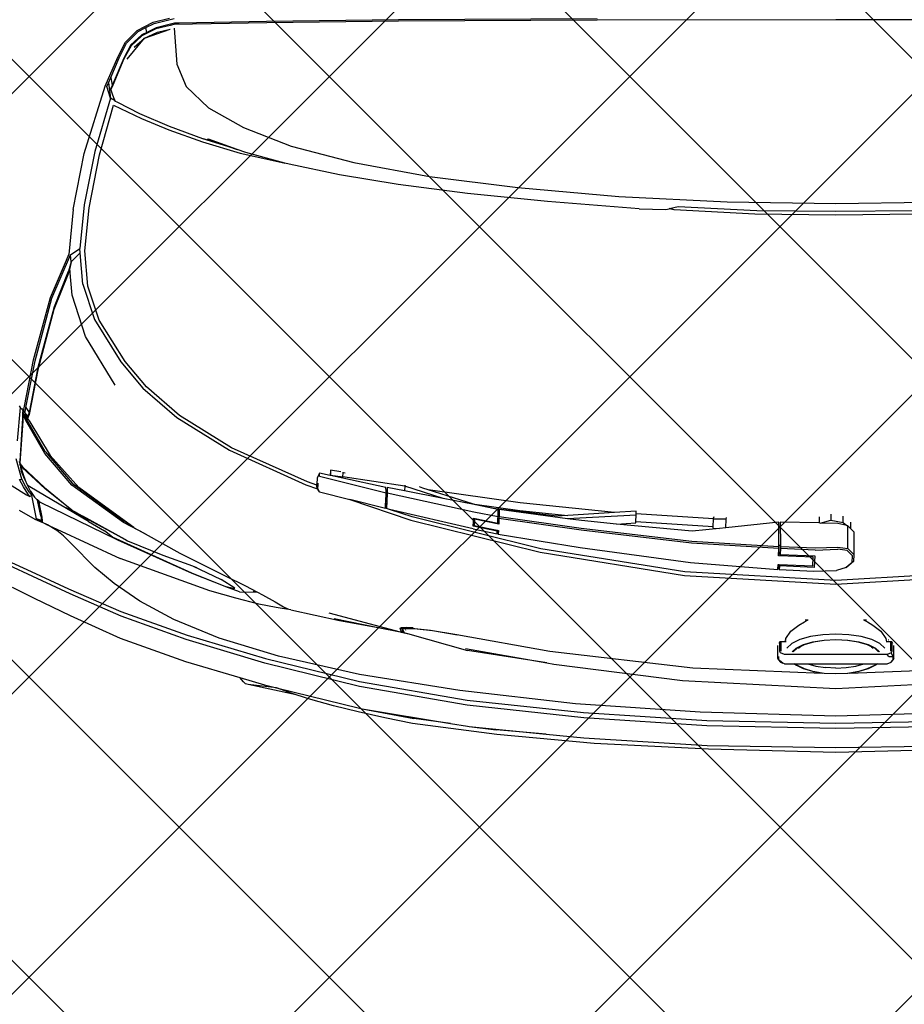
# Model space of a CAD drawing. Units: inches. Extents: x 2167 to 2589, y 1680 to 2489.
# Tile 4 of 38: x 2262.53 to 2283.35, y 1703.49 to 1726.68. Entities that reach past the tile are written whole.
import ezdxf

# ---------------------------------------------------------------- set-up
doc = ezdxf.new("R2010")
doc.units = ezdxf.units.IN
doc.header["$MEASUREMENT"] = 0
doc.layers.get('0').update_dxf_attribs({"color": 250})
for name, color, linetype, lineweight in [('A-ANNO-DIMS', 2, 'Continuous', 18), ('C-PRKG-VEHS', 8, 'Continuous', 13), ('L-PVMT-PATT', 252, 'Continuous', 13)]:
    doc.layers.add(name, color=color, linetype=linetype, lineweight=lineweight)
doc.layers.add('Edges', color=250, linetype='Continuous')
doc.styles.get("Standard").update_dxf_attribs({"font": 'arial.ttf'})
doc.dimstyles.get("Standard").update_dxf_attribs({"dimtxt": 7, "dimasz": 0.18, "dimexe": 0.18, "dimexo": 0.0625, "dimgap": 0.09, "dimtad": 0, "dimtih": 1, "dimtoh": 1, "dimdec": 1, "dimzin": 0, "dimdsep": 46, "dimlunit": 3, "dimtxsty": 'Standard', "dimcen": 0.09, "dimadec": 0, "dimazin": 0, "dimtfac": 1, "dimtdec": 1, "dimtofl": 0, "dimtmove": 0, "dimatfit": 3, "dimfxl": 1, "dimtolj": 1, "dimtzin": 0, "dimarcsym": 0})

# ---------------------------------------------------------------- blocks, each defined once
blk = doc.blocks.new('Nissan Qashqai pl')
at = {"layer": 'Edges'}
for p, q in [((11.05972, 12.11965), (11.05938, 11.92208)), ((11.5166, 12.04708), (11.52386, 11.92208)), ((11.52698, 11.92208), (11.51964, 12.0475)), ((11.61327, 11.92208), (11.60675, 12.04892)), ((11.60051, 11.93346), (11.59629, 12.04057)), ((11.63292, 12.0344), (11.63628, 11.92208)), ((11.64211, 11.92208), (11.63993, 12.02899)), ((11.64437, 12.02886), (11.64655, 11.92208)), ((11.66226, 11.92208), (11.66041, 12.02874)), ((11.66349, 12.02738), (11.66628, 11.92208)), ((11.21164, 11.92208), (11.21014, 12.01197)), ((11.21801, 11.92208), (11.21745, 11.98742)), ((11.22044, 11.98904), (11.22108, 11.92208)), ((11.57261, 11.96533), (11.57261, 11.96561)), ((11.57306, 11.96528), (11.57306, 11.96569)), ((11.57479, 11.96843), (11.57457, 11.96768)), ((11.58239, 11.96768), (11.57457, 11.96768)), ((11.57457, 11.96768), (11.57457, 11.96395)), ((11.57617, 11.96938), (11.57479, 11.96843)), ((11.57479, 11.96843), (11.58262, 11.96843)), ((11.58846, 11.97008), (11.57758, 11.97008)), ((11.58262, 11.96843), (11.58377, 11.96782)), ((11.58668, 11.96947), (11.58377, 11.96782)), ((11.58377, 11.96782), (11.58513, 11.96453)), ((11.58679, 11.96604), (11.58513, 11.96453)), ((11.58679, 11.96604), (11.58668, 11.96947)), ((11.58961, 11.96947), (11.58668, 11.96947)), ((11.58846, 11.97008), (11.58961, 11.96947)), ((11.5915, 11.96782), (11.58961, 11.96947)), ((11.5915, 11.96782), (11.59043, 11.96839)), ((11.59285, 11.96453), (11.5915, 11.96782)), ((11.56082, 11.95281), (11.56588, 11.95938)), ((11.56588, 11.95938), (11.57195, 11.96347)), ((11.57195, 11.96347), (11.57457, 11.96395)), ((11.57613, 11.95845), (11.57286, 11.95178)), ((11.57457, 11.96395), (11.57457, 11.96378)), ((11.57994, 11.96265), (11.57613, 11.95845)), ((11.57987, 11.95487), (11.58291, 11.95821)), ((11.58291, 11.95743), (11.58001, 11.95424)), ((11.58513, 11.96453), (11.58513, 11.87963)), ((11.59285, 11.95694), (11.59285, 11.96453)), ((11.55816, 11.94815), (11.56082, 11.95281)), ((11.57286, 11.95178), (11.57035, 11.94308)), ((11.57692, 11.94885), (11.57987, 11.95487)), ((11.57876, 11.95169), (11.57712, 11.94834)), ((11.58001, 11.95424), (11.57876, 11.95169)), ((11.57876, 11.95169), (11.57995, 11.953)), ((11.59285, 11.95694), (11.59412, 11.95487)), ((11.59285, 11.95657), (11.59285, 11.95694)), ((11.59319, 11.9559), (11.59285, 11.95657)), ((11.59285, 11.95626), (11.59285, 11.95657)), ((11.59285, 11.95626), (11.59319, 11.9559)), ((11.59285, 11.95549), (11.59285, 11.95626)), ((11.59398, 11.95424), (11.59285, 11.95549)), ((11.59285, 11.94526), (11.59285, 11.95549)), ((11.59319, 11.9559), (11.59412, 11.95487)), ((11.59688, 11.94834), (11.59398, 11.95424)), ((11.59412, 11.95487), (11.59707, 11.94885)), ((11.55654, 11.94509), (11.55639, 11.94749)), ((11.55654, 11.94509), (11.55816, 11.94815)), ((11.57035, 11.94308), (11.56877, 11.93295)), ((11.57324, 11.93188), (11.57466, 11.94101)), ((11.57466, 11.94101), (11.57692, 11.94885)), ((11.57712, 11.94834), (11.5749, 11.94065)), ((11.59285, 11.8989), (11.59285, 11.94526)), ((11.59478, 11.93858), (11.59285, 11.94526)), ((11.5991, 11.94065), (11.59688, 11.94834)), ((11.59707, 11.94885), (11.59933, 11.94101)), ((11.59933, 11.94101), (11.60051, 11.93346)), ((11.48106, 11.93457), (11.47554, 11.93456)), ((11.48106, 11.93457), (11.4786, 11.93206)), ((11.48349, 11.93703), (11.48106, 11.93457)), ((11.48349, 11.93703), (11.50222, 11.93704)), ((11.49744, 11.93207), (11.50222, 11.93704)), ((11.50349, 11.93588), (11.49907, 11.93132)), ((11.50222, 11.93704), (11.50812, 11.93671)), ((11.50889, 11.93558), (11.50349, 11.93588)), ((11.50812, 11.93671), (11.51287, 11.9312)), ((11.50889, 11.93558), (11.51321, 11.93053)), ((11.56877, 11.93295), (11.56823, 11.92208)), ((11.5749, 11.94065), (11.5735, 11.93169)), ((11.59602, 11.93062), (11.59478, 11.93858)), ((11.60049, 11.93169), (11.5991, 11.94065)), ((11.60051, 11.93346), (11.60076, 11.93188)), ((11.47578, 11.92803), (11.47062, 11.92803)), ((11.47398, 11.91798), (11.47578, 11.92803)), ((11.47578, 11.92803), (11.4784, 11.93124)), ((11.4784, 11.93124), (11.47657, 11.92368)), ((11.4786, 11.93206), (11.4784, 11.93124)), ((11.49744, 11.93207), (11.4786, 11.93206)), ((11.49621, 11.92369), (11.49744, 11.93207)), ((11.49907, 11.93132), (11.49795, 11.92364)), ((11.51321, 11.93053), (11.51287, 11.9312)), ((11.51321, 11.93053), (11.51543, 11.92267)), ((11.57275, 11.92208), (11.57324, 11.93188)), ((11.5735, 11.93169), (11.57302, 11.92208)), ((11.59645, 11.92208), (11.59602, 11.93062)), ((11.60097, 11.92208), (11.60049, 11.93169)), ((11.60076, 11.93188), (11.60124, 11.92208)), ((11.05938, 11.92208), (11.05972, 11.72451)), ((11.21014, 11.8322), (11.21164, 11.92208)), ((11.21745, 11.85674), (11.21801, 11.92208)), ((11.22108, 11.92208), (11.22044, 11.85512)), ((11.46896, 11.91798), (11.47398, 11.91798)), ((11.47622, 11.90912), (11.47398, 11.91798)), ((11.47657, 11.92368), (11.47622, 11.90912)), ((11.49689, 11.90495), (11.49621, 11.92369)), ((11.49859, 11.9049), (11.49795, 11.92364)), ((11.51606, 11.90392), (11.51543, 11.92267)), ((11.52386, 11.92208), (11.5166, 11.79708)), ((11.51964, 11.79666), (11.52698, 11.92208)), ((11.56823, 11.92208), (11.56877, 11.91121)), ((11.57324, 11.91228), (11.57275, 11.92208)), ((11.57302, 11.92208), (11.5735, 11.91247)), ((11.59645, 11.92208), (11.59602, 11.91354)), ((11.60049, 11.91247), (11.60097, 11.92208)), ((11.60124, 11.92208), (11.60076, 11.91228)), ((11.60675, 11.79524), (11.61327, 11.92208)), ((11.63628, 11.92208), (11.63292, 11.80976)), ((11.63993, 11.81518), (11.64211, 11.92208)), ((11.64655, 11.92208), (11.64437, 11.8153)), ((11.66041, 11.81542), (11.66226, 11.92208)), ((11.66628, 11.92208), (11.66349, 11.81678)), ((11.47102, 11.90825), (11.4762, 11.90826)), ((11.4762, 11.90826), (11.47542, 11.87608)), ((11.47622, 11.90912), (11.4762, 11.90826)), ((11.56877, 11.91121), (11.57035, 11.90108)), ((11.57466, 11.90315), (11.57324, 11.91228)), ((11.5735, 11.91247), (11.5749, 11.90351)), ((11.59478, 11.90558), (11.59602, 11.91354)), ((11.59629, 11.80359), (11.60051, 11.91071)), ((11.5991, 11.90351), (11.60049, 11.91247)), ((11.60051, 11.91071), (11.59933, 11.90315)), ((11.60076, 11.91228), (11.60051, 11.91071)), ((11.49565, 11.87616), (11.49689, 11.90495)), ((11.49859, 11.9049), (11.49735, 11.87612)), ((11.50223, 11.8759), (11.50346, 11.90468)), ((11.50462, 11.90341), (11.50341, 11.87505)), ((11.50346, 11.90468), (11.51299, 11.90415)), ((11.51177, 11.90301), (11.50462, 11.90341)), ((11.51058, 11.87508), (11.51177, 11.90301)), ((11.51299, 11.90415), (11.51176, 11.87537)), ((11.51483, 11.87514), (11.51606, 11.90392)), ((11.57035, 11.90108), (11.57286, 11.89238)), ((11.57692, 11.89531), (11.57466, 11.90315)), ((11.5749, 11.90351), (11.57712, 11.89582)), ((11.59285, 11.8989), (11.59478, 11.90558)), ((11.59688, 11.89582), (11.5991, 11.90351)), ((11.59933, 11.90315), (11.59707, 11.89531)), ((11.55639, 11.89667), (11.55654, 11.89907)), ((11.55816, 11.89601), (11.55654, 11.89907)), ((11.56082, 11.89135), (11.55816, 11.89601)), ((11.57286, 11.89238), (11.57613, 11.88571)), ((11.57987, 11.88929), (11.57692, 11.89531)), ((11.57712, 11.89582), (11.57876, 11.89248)), ((11.57995, 11.89116), (11.57876, 11.89248)), ((11.57876, 11.89248), (11.58001, 11.88992)), ((11.59285, 11.88868), (11.59285, 11.8989)), ((11.59398, 11.88992), (11.59688, 11.89582)), ((11.59707, 11.89531), (11.59412, 11.88929)), ((11.56588, 11.88478), (11.56082, 11.89135)), ((11.57195, 11.88069), (11.56588, 11.88478)), ((11.57613, 11.88571), (11.57994, 11.88151)), ((11.58291, 11.88595), (11.57987, 11.88929)), ((11.58001, 11.88992), (11.58291, 11.88673)), ((11.59285, 11.88868), (11.59398, 11.88992)), ((11.59285, 11.88722), (11.59412, 11.88929)), ((11.59285, 11.8879), (11.59285, 11.88868)), ((11.59285, 11.88759), (11.59319, 11.88827)), ((11.59319, 11.88827), (11.59285, 11.8879)), ((11.59285, 11.88759), (11.59285, 11.8879)), ((11.59285, 11.88722), (11.59285, 11.88759)), ((11.59285, 11.87963), (11.59285, 11.88722)), ((11.59412, 11.88929), (11.59319, 11.88827)), ((11.47542, 11.87608), (11.49451, 11.87616)), ((11.49449, 11.87502), (11.49451, 11.87616)), ((11.49451, 11.87616), (11.49565, 11.87616)), ((11.49565, 11.87616), (11.49735, 11.87612)), ((11.49735, 11.87612), (11.50223, 11.8759)), ((11.57261, 11.88057), (11.57195, 11.88069)), ((11.57261, 11.88057), (11.57261, 11.88076)), ((11.57306, 11.88049), (11.57261, 11.88057)), ((11.57306, 11.88049), (11.57306, 11.88081)), ((11.57457, 11.88021), (11.57306, 11.88049)), ((11.57457, 11.88096), (11.57457, 11.88021)), ((11.57457, 11.88021), (11.57457, 11.87648)), ((11.57457, 11.87648), (11.58239, 11.87648)), ((11.57457, 11.87648), (11.57479, 11.87573)), ((11.58262, 11.87573), (11.57479, 11.87573)), ((11.57479, 11.87573), (11.57617, 11.87478)), ((11.58377, 11.87635), (11.58262, 11.87573)), ((11.58513, 11.87963), (11.58377, 11.87635)), ((11.58961, 11.87469), (11.5915, 11.87635)), ((11.59043, 11.87577), (11.58961, 11.87469)), ((11.59221, 11.87812), (11.59043, 11.87577)), ((11.59043, 11.87577), (11.5915, 11.87635)), ((11.5915, 11.87635), (11.59221, 11.87812)), ((11.59285, 11.87963), (11.59221, 11.87812)), ((11.49563, 11.87496), (11.47539, 11.87488)), ((11.47539, 11.87488), (11.4801, 11.83099)), ((11.49133, 11.80278), (11.49563, 11.87496)), ((11.49732, 11.87492), (11.49295, 11.80271)), ((11.50341, 11.87505), (11.49449, 11.87502)), ((11.49732, 11.87492), (11.49563, 11.87496)), ((11.50339, 11.87463), (11.49732, 11.87492)), ((11.50341, 11.87505), (11.50339, 11.87463)), ((11.50884, 11.80182), (11.5148, 11.87394)), ((11.51054, 11.87423), (11.51058, 11.87508)), ((11.5148, 11.87394), (11.51054, 11.87423)), ((11.51472, 11.8751), (11.51058, 11.87508)), ((11.51176, 11.87537), (11.51472, 11.87515)), ((11.51472, 11.87515), (11.51472, 11.8751)), ((11.51472, 11.87515), (11.51483, 11.87514)), ((11.51483, 11.87514), (11.51472, 11.8751)), ((11.58846, 11.87408), (11.57758, 11.87408)), ((11.58668, 11.87469), (11.58961, 11.87469)), ((11.58961, 11.87469), (11.58846, 11.87408)), ((11.2139, 11.7914), (11.21745, 11.85674)), ((11.22044, 11.85512), (11.21682, 11.78816)), ((11.20565, 11.74231), (11.21014, 11.8322)), ((11.47305, 11.83139), (11.47165, 11.83144)), ((11.47305, 11.83139), (11.473, 11.82087)), ((11.4801, 11.83099), (11.47305, 11.83139)), ((11.4801, 11.83099), (11.48065, 11.82584)), ((11.47281, 11.82086), (11.46872, 11.75675)), ((11.47111, 11.82093), (11.47189, 11.82089)), ((11.47281, 11.82086), (11.47189, 11.82089)), ((11.473, 11.82087), (11.47281, 11.82086)), ((11.47916, 11.8205), (11.473, 11.82087)), ((11.47508, 11.75641), (11.47919, 11.82046)), ((11.47919, 11.82046), (11.47916, 11.8205)), ((11.48062, 11.82044), (11.47919, 11.82046)), ((11.48062, 11.82044), (11.48065, 11.82584)), ((11.48065, 11.82584), (11.4831, 11.803)), ((11.63327, 11.71316), (11.63993, 11.81518)), ((11.64437, 11.8153), (11.63768, 11.7134)), ((11.65425, 11.71357), (11.66041, 11.81542)), ((11.66349, 11.81678), (11.65888, 11.72193)), ((11.4831, 11.803), (11.47707, 11.74042)), ((11.4805, 11.71128), (11.49133, 11.80278)), ((11.49295, 11.80271), (11.48212, 11.71121)), ((11.58235, 11.68521), (11.59629, 11.80359)), ((11.63292, 11.80976), (11.62604, 11.70665)), ((11.49642, 11.71041), (11.50884, 11.80182)), ((11.5166, 11.79708), (11.49761, 11.67796)), ((11.50045, 11.6772), (11.51964, 11.79666)), ((11.5932, 11.68852), (11.60675, 11.79524)), ((11.21579, 11.78424), (11.2139, 11.7914)), ((11.21682, 11.78816), (11.21579, 11.78424)), ((11.21682, 11.78816), (11.21585, 11.78401)), ((11.21585, 11.78401), (11.21579, 11.78424)), ((11.21658, 11.78121), (11.21585, 11.78401)), ((11.21586, 11.75915), (11.21658, 11.78121)), ((11.21586, 11.75915), (11.20997, 11.68347)), ((11.46872, 11.75675), (11.46649, 11.75682)), ((11.46649, 11.75682), (11.46757, 11.73891)), ((11.46975, 11.75671), (11.46872, 11.75675)), ((11.46975, 11.75671), (11.47273, 11.69994)), ((11.47508, 11.75641), (11.46975, 11.75671)), ((11.47611, 11.75636), (11.47508, 11.75641)), ((11.47707, 11.74042), (11.47611, 11.75636)), ((11.19842, 11.65867), (11.20565, 11.74231)), ((11.46757, 11.73891), (11.45941, 11.6607)), ((11.46757, 11.73891), (11.46992, 11.70014)), ((11.47707, 11.74042), (11.47428, 11.71144)), ((11.0586, 11.72441), (11.05947, 11.55994)), ((11.05972, 11.72451), (11.06059, 11.56009)), ((11.65888, 11.72193), (11.65143, 11.64152)), ((11.6229, 11.61679), (11.63327, 11.71316)), ((11.63768, 11.7134), (11.62719, 11.61693)), ((11.65114, 11.68233), (11.65425, 11.71357)), ((11.47094, 11.64327), (11.4805, 11.71128)), ((11.48212, 11.71121), (11.47257, 11.6432)), ((11.47428, 11.71144), (11.47273, 11.69994)), ((11.48539, 11.64249), (11.49642, 11.71041)), ((11.62604, 11.70665), (11.61495, 11.61084)), ((11.47273, 11.69994), (11.46512, 11.64343)), ((11.46576, 11.66035), (11.46992, 11.70014)), ((11.46992, 11.70014), (11.47047, 11.69095)), ((11.47047, 11.69095), (11.46419, 11.63849)), ((11.59218, 11.68277), (11.5932, 11.68852)), ((11.20997, 11.68347), (11.2033, 11.61723)), ((11.56846, 11.60829), (11.58235, 11.68521)), ((11.58021, 11.61555), (11.59218, 11.68277)), ((11.59218, 11.68277), (11.58179, 11.61717)), ((11.64478, 11.61839), (11.65114, 11.68233)), ((11.65114, 11.68233), (11.64749, 11.64092)), ((11.49761, 11.67796), (11.47115, 11.57128)), ((11.47375, 11.5702), (11.50045, 11.6772)), ((11.18907, 11.58559), (11.19842, 11.65867)), ((11.45941, 11.6607), (11.44866, 11.58459)), ((11.46024, 11.62121), (11.46576, 11.66035)), ((11.46505, 11.64255), (11.46419, 11.63849)), ((11.46792, 11.64248), (11.46505, 11.64255)), ((11.46512, 11.64343), (11.46801, 11.64335)), ((11.46687, 11.62247), (11.47088, 11.64239)), ((11.46801, 11.64335), (11.46792, 11.64248)), ((11.47088, 11.64239), (11.46792, 11.64248)), ((11.46801, 11.64335), (11.47094, 11.64327)), ((11.47252, 11.64233), (11.47088, 11.64239)), ((11.47094, 11.64327), (11.47257, 11.6432)), ((11.47212, 11.62223), (11.47625, 11.64214)), ((11.47439, 11.64223), (11.47252, 11.64233)), ((11.47257, 11.6432), (11.47449, 11.6431)), ((11.47727, 11.64296), (11.47315, 11.62305)), ((11.47439, 11.64223), (11.47449, 11.6431)), ((11.47625, 11.64214), (11.47439, 11.64223)), ((11.47449, 11.6431), (11.47727, 11.64296)), ((11.47827, 11.62277), (11.48226, 11.64167)), ((11.48298, 11.64165), (11.47879, 11.62186)), ((11.48098, 11.62171), (11.48532, 11.64161)), ((11.48226, 11.64167), (11.48244, 11.64254)), ((11.48226, 11.64167), (11.48298, 11.64165)), ((11.48244, 11.64254), (11.48247, 11.64267)), ((11.48535, 11.64246), (11.48244, 11.64254)), ((11.48247, 11.64267), (11.48535, 11.64246)), ((11.483, 11.64176), (11.48298, 11.64165)), ((11.48532, 11.64161), (11.483, 11.64176)), ((11.48539, 11.64249), (11.48535, 11.64246)), ((11.65143, 11.64152), (11.64217, 11.57162)), ((11.64478, 11.61839), (11.64749, 11.64092)), ((11.46419, 11.63849), (11.46114, 11.62406)), ((11.46114, 11.62406), (11.46024, 11.62121)), ((11.46114, 11.62406), (11.46083, 11.62261)), ((11.47315, 11.62305), (11.47515, 11.62294)), ((11.47495, 11.62207), (11.47515, 11.62294)), ((11.47515, 11.62294), (11.47827, 11.62277)), ((11.2033, 11.61723), (11.19582, 11.55976)), ((11.46024, 11.62121), (11.44866, 11.58459)), ((11.45125, 11.55073), (11.46687, 11.62247)), ((11.46083, 11.62261), (11.45585, 11.5969)), ((11.48098, 11.62171), (11.4649, 11.55261)), ((11.47495, 11.62207), (11.47212, 11.62223)), ((11.47879, 11.62186), (11.47495, 11.62207)), ((11.56776, 11.56755), (11.58179, 11.61717)), ((11.60765, 11.5276), (11.6229, 11.61679)), ((11.62719, 11.61693), (11.61178, 11.52762)), ((11.64227, 11.603), (11.64462, 11.61709)), ((11.64462, 11.61709), (11.64478, 11.61839)), ((11.56499, 11.58644), (11.56846, 11.60829)), ((11.56905, 11.60888), (11.56563, 11.58822)), ((11.61495, 11.61084), (11.6016, 11.52761)), ((11.63012, 11.53004), (11.64227, 11.603)), ((11.64227, 11.603), (11.63807, 11.5726)), ((11.45585, 11.5969), (11.44582, 11.56516)), ((11.45585, 11.5969), (11.44965, 11.56495)), ((11.17758, 11.52307), (11.18907, 11.58559)), ((11.44866, 11.58459), (11.44723, 11.58007)), ((11.56356, 11.57357), (11.56499, 11.58644)), ((11.56563, 11.58822), (11.56415, 11.57536)), ((11.44723, 11.58007), (11.44639, 11.57739)), ((11.56415, 11.57536), (11.56375, 11.56794)), ((11.45676, 11.51971), (11.47375, 11.5702)), ((11.47115, 11.57128), (11.4649, 11.55261)), ((11.56255, 11.56701), (11.56268, 11.56956)), ((11.56271, 11.56245), (11.56255, 11.56701)), ((11.56268, 11.56956), (11.56259, 11.5697)), ((11.56268, 11.56956), (11.5628, 11.57206)), ((11.56335, 11.56843), (11.56268, 11.56956)), ((11.56325, 11.56586), (11.56335, 11.56843)), ((11.56334, 11.56271), (11.56325, 11.56586)), ((11.56335, 11.56843), (11.56356, 11.57357)), ((11.56368, 11.56788), (11.56335, 11.56843)), ((11.56375, 11.56794), (11.56392, 11.56325)), ((11.56487, 11.5659), (11.56469, 11.5662)), ((11.56704, 11.56455), (11.56739, 11.56625)), ((11.56712, 11.56458), (11.56763, 11.56708)), ((11.56717, 11.5646), (11.56763, 11.56708)), ((11.56745, 11.56646), (11.56739, 11.56625)), ((11.56763, 11.56708), (11.56776, 11.56755)), ((11.63012, 11.53004), (11.63807, 11.5726)), ((11.64217, 11.57162), (11.63751, 11.54857)), ((11.05947, 11.55994), (11.06074, 11.45082)), ((11.06059, 11.56009), (11.06182, 11.4509)), ((11.19582, 11.55976), (11.18773, 11.51111)), ((11.44575, 11.56516), (11.43801, 11.51398)), ((11.4448, 11.5652), (11.44575, 11.56516)), ((11.44575, 11.56516), (11.44582, 11.56516)), ((11.44582, 11.56516), (11.44965, 11.56495)), ((11.44965, 11.56495), (11.44685, 11.5505)), ((11.55053, 11.5023), (11.56648, 11.56144)), ((11.56334, 11.56271), (11.56271, 11.56245)), ((11.56338, 11.56129), (11.56271, 11.56245)), ((11.56273, 11.5431), (11.56648, 11.56144)), ((11.56609, 11.56386), (11.56334, 11.56271)), ((11.56338, 11.56129), (11.56334, 11.56271)), ((11.56583, 11.56223), (11.56338, 11.56129)), ((11.56392, 11.56325), (11.56429, 11.56338)), ((11.56429, 11.56338), (11.56596, 11.56408)), ((11.56609, 11.56386), (11.56583, 11.56223)), ((11.56616, 11.56236), (11.56583, 11.56223)), ((11.56596, 11.56408), (11.56616, 11.56417)), ((11.56609, 11.56386), (11.56596, 11.56408)), ((11.56613, 11.56388), (11.56609, 11.56386)), ((11.56618, 11.56418), (11.56613, 11.56388)), ((11.56613, 11.56388), (11.56616, 11.56417)), ((11.56613, 11.56388), (11.56645, 11.5641)), ((11.56665, 11.56424), (11.56616, 11.56236)), ((11.56616, 11.56417), (11.56618, 11.56418)), ((11.56616, 11.56236), (11.56645, 11.5641)), ((11.56661, 11.56253), (11.56616, 11.56236)), ((11.56618, 11.56418), (11.56648, 11.56431)), ((11.56645, 11.5641), (11.56648, 11.56431)), ((11.56645, 11.5641), (11.56665, 11.56424)), ((11.56648, 11.56431), (11.56669, 11.5644)), ((11.56679, 11.56261), (11.56648, 11.56144)), ((11.56661, 11.56253), (11.56704, 11.56455)), ((11.56671, 11.56257), (11.56661, 11.56253)), ((11.56665, 11.56424), (11.56688, 11.56448)), ((11.56669, 11.5644), (11.56665, 11.56424)), ((11.56669, 11.5644), (11.56688, 11.56448)), ((11.56671, 11.56257), (11.56712, 11.56458)), ((11.56679, 11.56261), (11.56671, 11.56257)), ((11.56717, 11.5646), (11.56679, 11.56261)), ((11.56688, 11.56448), (11.56704, 11.56455)), ((11.56704, 11.56455), (11.56712, 11.56458)), ((11.56712, 11.56458), (11.56717, 11.5646)), ((11.43747, 11.49463), (11.45125, 11.54985)), ((11.44684, 11.54963), (11.43914, 11.51392)), ((11.44983, 11.54978), (11.44684, 11.54963)), ((11.44685, 11.5505), (11.44997, 11.55066)), ((11.44983, 11.54978), (11.44997, 11.55066)), ((11.45125, 11.54985), (11.44983, 11.54978)), ((11.44997, 11.55066), (11.45125, 11.55073)), ((11.45125, 11.55073), (11.4529, 11.55066)), ((11.4529, 11.54978), (11.45125, 11.54985)), ((11.4529, 11.55066), (11.45711, 11.55045)), ((11.45711, 11.54958), (11.4529, 11.54978)), ((11.45711, 11.55045), (11.45994, 11.5503)), ((11.46197, 11.5493), (11.45711, 11.54958)), ((11.45983, 11.54978), (11.45994, 11.5503)), ((11.46402, 11.54999), (11.45983, 11.54978)), ((11.45994, 11.5503), (11.46197, 11.55018)), ((11.46197, 11.55018), (11.46404, 11.55004)), ((11.46375, 11.54918), (11.46197, 11.5493)), ((11.46402, 11.54999), (11.46375, 11.54918)), ((11.46404, 11.55004), (11.46402, 11.54999)), ((11.46423, 11.55), (11.46402, 11.54999)), ((11.46404, 11.55004), (11.46423, 11.55)), ((11.46423, 11.55), (11.46424, 11.55003)), ((11.4643, 11.55002), (11.46423, 11.55)), ((11.4649, 11.55261), (11.4643, 11.55002)), ((11.46429, 11.54915), (11.45676, 11.51971)), ((11.46429, 11.54915), (11.46375, 11.54918)), ((11.55533, 11.50682), (11.56273, 11.5431)), ((11.55707, 11.51104), (11.56273, 11.5431)), ((11.63751, 11.54857), (11.63276, 11.52672)), ((11.6016, 11.52761), (11.58664, 11.46068)), ((11.58843, 11.44985), (11.60765, 11.5276)), ((11.61178, 11.52762), (11.59225, 11.44945)), ((11.61272, 11.45895), (11.62966, 11.52759)), ((11.63276, 11.52672), (11.62771, 11.50627)), ((11.62966, 11.52759), (11.63012, 11.53004)), ((11.16395, 11.47112), (11.17758, 11.52307)), ((11.45032, 11.49453), (11.45676, 11.51971)), ((11.18773, 11.51111), (11.17906, 11.46956)), ((11.43371, 11.51238), (11.43251, 11.50378)), ((11.43475, 11.51409), (11.43403, 11.51411)), ((11.43501, 11.51584), (11.43475, 11.51409)), ((11.43801, 11.51398), (11.43475, 11.51409)), ((11.4382, 11.51397), (11.43676, 11.50364)), ((11.43914, 11.51392), (11.43692, 11.50363)), ((11.4382, 11.51397), (11.43801, 11.51398)), ((11.43914, 11.51392), (11.4382, 11.51397)), ((11.54814, 11.47101), (11.55707, 11.51104)), ((11.43251, 11.50378), (11.43676, 11.50364)), ((11.43251, 11.50378), (11.4369, 11.50353)), ((11.4369, 11.50353), (11.435, 11.49469)), ((11.43676, 11.50364), (11.43692, 11.50363)), ((11.43692, 11.50363), (11.4369, 11.50353)), ((11.62771, 11.50627), (11.62241, 11.48743)), ((11.435, 11.49469), (11.43896, 11.49272)), ((11.43747, 11.49463), (11.435, 11.49469)), ((11.43896, 11.49272), (11.44373, 11.49245)), ((11.44474, 11.49242), (11.44218, 11.48476)), ((11.44507, 11.49341), (11.44316, 11.49351)), ((11.44373, 11.49245), (11.44491, 11.49291)), ((11.44474, 11.49242), (11.44373, 11.49245)), ((11.44453, 11.48334), (11.44778, 11.49299)), ((11.44491, 11.49291), (11.44474, 11.49242)), ((11.4462, 11.49239), (11.44474, 11.49242)), ((11.44507, 11.49341), (11.44491, 11.49291)), ((11.44491, 11.49291), (11.44606, 11.49335)), ((11.44606, 11.49335), (11.44507, 11.49341)), ((11.44786, 11.49325), (11.44606, 11.49335)), ((11.44786, 11.49325), (11.4462, 11.49239)), ((11.44778, 11.49299), (11.4462, 11.49239)), ((11.45018, 11.49392), (11.44778, 11.49299)), ((11.44794, 11.49325), (11.44786, 11.49325)), ((11.45032, 11.49453), (11.44794, 11.49325)), ((11.45018, 11.49392), (11.45032, 11.49453)), ((11.44218, 11.48476), (11.41383, 11.42186)), ((11.62241, 11.48743), (11.61848, 11.47528)), ((11.41588, 11.41997), (11.44453, 11.48334)), ((11.14869, 11.43161), (11.16395, 11.47112)), ((11.17906, 11.46956), (11.17808, 11.46592)), ((11.54554, 11.46484), (11.54721, 11.46841)), ((11.54814, 11.47101), (11.54666, 11.46197)), ((11.61848, 11.47528), (11.61008, 11.43562)), ((11.61742, 11.47198), (11.61272, 11.45895)), ((11.61848, 11.47528), (11.61742, 11.47198)), ((11.17808, 11.46592), (11.1694, 11.43374)), ((11.1699, 11.42889), (11.17797, 11.4652)), ((11.17797, 11.4652), (11.17808, 11.46592)), ((11.54162, 11.45783), (11.54554, 11.46484)), ((11.54666, 11.46197), (11.54611, 11.45874)), ((11.58664, 11.46068), (11.57152, 11.41151)), ((11.53572, 11.44731), (11.54162, 11.45783)), ((11.54611, 11.45874), (11.54336, 11.44449)), ((11.61272, 11.45895), (11.61008, 11.43562)), ((11.61028, 11.44915), (11.61272, 11.45895)), ((11.06074, 11.45082), (11.06214, 11.37845)), ((11.06182, 11.4509), (11.06324, 11.37414)), ((11.53354, 11.44315), (11.53572, 11.44731)), ((11.54336, 11.44449), (11.53855, 11.42543)), ((11.56912, 11.38501), (11.58843, 11.44985)), ((11.59225, 11.44945), (11.57263, 11.38419)), ((11.60419, 11.42861), (11.61028, 11.44915)), ((11.52833, 11.43321), (11.53335, 11.4428)), ((11.53261, 11.43965), (11.5333, 11.44225)), ((11.53313, 11.42848), (11.53354, 11.44315)), ((11.5333, 11.44225), (11.53335, 11.4428)), ((11.53335, 11.4428), (11.53354, 11.44315)), ((11.61008, 11.43562), (11.60938, 11.43347)), ((11.1323, 11.40268), (11.14869, 11.43161)), ((11.16047, 11.39766), (11.1699, 11.42889)), ((11.1694, 11.43374), (11.1668, 11.42651)), ((11.5202, 11.41712), (11.52833, 11.43321)), ((11.53313, 11.42848), (11.52922, 11.417)), ((11.59084, 11.38361), (11.60419, 11.42861)), ((11.60772, 11.43162), (11.60419, 11.42861)), ((11.60938, 11.43347), (11.60772, 11.43162)), ((11.15764, 11.39828), (11.16426, 11.41918)), ((11.15766, 11.39771), (11.16426, 11.41918)), ((11.1668, 11.42651), (11.1582, 11.40259)), ((11.16426, 11.41918), (11.15826, 11.40186)), ((11.16426, 11.41918), (11.1668, 11.42651)), ((11.41383, 11.42186), (11.38718, 11.37878)), ((11.38877, 11.37638), (11.41588, 11.41997)), ((11.53009, 11.42439), (11.52299, 11.41307)), ((11.52855, 11.41625), (11.53022, 11.42324)), ((11.53022, 11.42324), (11.53009, 11.42439)), ((11.53855, 11.42543), (11.53253, 11.4038)), ((11.50131, 11.37908), (11.5202, 11.41712)), ((11.5118, 11.38938), (11.52299, 11.41307)), ((11.52922, 11.417), (11.51787, 11.38901)), ((11.51787, 11.38901), (11.52855, 11.41625)), ((11.57152, 11.41151), (11.55624, 11.37411)), ((11.11477, 11.38434), (11.1323, 11.40268)), ((11.53253, 11.4038), (11.50574, 11.32965)), ((11.14751, 11.37001), (11.15766, 11.39771)), ((11.15051, 11.36998), (11.16047, 11.39766)), ((11.51787, 11.38901), (11.48801, 11.32337)), ((11.49005, 11.3275), (11.51787, 11.38901)), ((11.50277, 11.36495), (11.5118, 11.38938)), ((11.5118, 11.38938), (11.51304, 11.39274)), ((11.06214, 11.37845), (11.06222, 11.37449)), ((11.09618, 11.37663), (11.11477, 11.38434)), ((11.38718, 11.37878), (11.3635, 11.35125)), ((11.48518, 11.35017), (11.50131, 11.37908)), ((11.54963, 11.33002), (11.56912, 11.38501)), ((11.57263, 11.38419), (11.5535, 11.33028)), ((11.57164, 11.32969), (11.59084, 11.38361)), ((11.06139, 11.35691), (11.05807, 11.37037)), ((11.06236, 11.3576), (11.05822, 11.37418)), ((11.06222, 11.37449), (11.06303, 11.37135)), ((11.06303, 11.37135), (11.06594, 11.3594)), ((11.06324, 11.37414), (11.06408, 11.37085)), ((11.06408, 11.37085), (11.06692, 11.35921)), ((11.06624, 11.37435), (11.09618, 11.37663)), ((11.06961, 11.36056), (11.0671, 11.37109)), ((11.07472, 11.34981), (11.0671, 11.37109)), ((11.13692, 11.34555), (11.14751, 11.37001)), ((11.14123, 11.34726), (11.15051, 11.36998)), ((11.36451, 11.34835), (11.38877, 11.37638)), ((11.55624, 11.37411), (11.54097, 11.34593)), ((11.49086, 11.33567), (11.50277, 11.36495)), ((11.06818, 11.34377), (11.06139, 11.35691)), ((11.06584, 11.35092), (11.06236, 11.3576)), ((11.06594, 11.3594), (11.06978, 11.35164)), ((11.06692, 11.35921), (11.0727, 11.34754)), ((11.07472, 11.34981), (11.06961, 11.36056)), ((11.06978, 11.35164), (11.06584, 11.35092)), ((11.06918, 11.34452), (11.06584, 11.35092)), ((11.06978, 11.35164), (11.07183, 11.3475)), ((11.07183, 11.3475), (11.08018, 11.33842)), ((11.0727, 11.34754), (11.0809, 11.33858)), ((11.08206, 11.34125), (11.07472, 11.34981)), ((11.092, 11.33548), (11.07472, 11.34981)), ((11.12767, 11.32749), (11.13692, 11.34555)), ((11.13017, 11.32416), (11.14123, 11.34726)), ((11.3635, 11.35125), (11.34251, 11.3336)), ((11.34283, 11.33026), (11.36451, 11.34835)), ((11.48518, 11.35017), (11.4758, 11.33232)), ((11.48012, 11.34111), (11.48518, 11.35017)), ((11.54097, 11.34593), (11.52646, 11.32473)), ((11.07787, 11.3339), (11.06818, 11.34377)), ((11.07866, 11.33492), (11.06918, 11.34452)), ((11.08018, 11.33842), (11.09121, 11.33249)), ((11.0809, 11.33858), (11.09174, 11.33271)), ((11.48005, 11.341), (11.44669, 11.29536)), ((11.47876, 11.33901), (11.47454, 11.33252)), ((11.47876, 11.33901), (11.48005, 11.341)), ((11.48005, 11.341), (11.48012, 11.34111)), ((11.09022, 11.32753), (11.07787, 11.3339)), ((11.09081, 11.32882), (11.07866, 11.33492)), ((11.09121, 11.33249), (11.1138, 11.3229)), ((11.09174, 11.33271), (11.11486, 11.323)), ((11.30757, 11.30833), (11.34283, 11.33026)), ((11.34251, 11.3336), (11.3082, 11.31215)), ((11.44331, 11.28988), (11.47454, 11.33252)), ((11.4758, 11.33232), (11.44474, 11.28965)), ((11.46332, 11.28473), (11.48966, 11.33337)), ((11.47038, 11.29841), (11.49086, 11.33567)), ((11.47038, 11.29841), (11.48966, 11.33337)), ((11.48133, 11.27727), (11.50574, 11.32965)), ((11.48966, 11.33337), (11.49086, 11.33567)), ((11.53062, 11.28691), (11.54963, 11.33002)), ((11.5535, 11.33028), (11.53487, 11.28826)), ((11.55274, 11.28821), (11.57164, 11.32969)), ((11.11439, 11.31711), (11.09022, 11.32753)), ((11.10704, 11.32181), (11.09081, 11.32882)), ((11.10704, 11.32181), (11.1138, 11.3229)), ((11.11164, 11.31982), (11.10704, 11.32181)), ((11.11164, 11.31982), (11.1244, 11.32146)), ((11.1138, 11.3229), (11.11393, 11.32284)), ((11.11393, 11.32284), (11.1164, 11.32172)), ((11.1244, 11.32146), (11.11467, 11.31851)), ((11.11486, 11.323), (11.1172, 11.32196)), ((11.1164, 11.32172), (11.1172, 11.32196)), ((11.11744, 11.32189), (11.1164, 11.32172)), ((11.1172, 11.32196), (11.11744, 11.32189)), ((11.11744, 11.32189), (11.11997, 11.32267)), ((11.11997, 11.32267), (11.12459, 11.32429)), ((11.12604, 11.32481), (11.1244, 11.32146)), ((11.1244, 11.32146), (11.12591, 11.32476)), ((11.1244, 11.32146), (11.16836, 11.30873)), ((11.12459, 11.32429), (11.12591, 11.32476)), ((11.12466, 11.32442), (11.12595, 11.32486)), ((11.12478, 11.32467), (11.12595, 11.32486)), ((11.12595, 11.32486), (11.1251, 11.3253)), ((11.12591, 11.32476), (11.12595, 11.32486)), ((11.12591, 11.32476), (11.12604, 11.32481)), ((11.12595, 11.32486), (11.12626, 11.32554)), ((11.12595, 11.32486), (11.12607, 11.32488)), ((11.12604, 11.32481), (11.12645, 11.32495)), ((11.12607, 11.32488), (11.12604, 11.32481)), ((11.12631, 11.32537), (11.12607, 11.32488)), ((11.12607, 11.32488), (11.12645, 11.32495)), ((11.12645, 11.32495), (11.12767, 11.32749)), ((11.17121, 11.31245), (11.13017, 11.32416)), ((11.36192, 11.32544), (11.32179, 11.30083)), ((11.45883, 11.26345), (11.48954, 11.32636)), ((11.48801, 11.32337), (11.48281, 11.31653)), ((11.48983, 11.32694), (11.48954, 11.32636)), ((11.48983, 11.32694), (11.49005, 11.3275)), ((11.52646, 11.32473), (11.51313, 11.30854)), ((11.11467, 11.31851), (11.11164, 11.31982)), ((11.17021, 11.29978), (11.11439, 11.31711)), ((11.47499, 11.30324), (11.48281, 11.31653)), ((11.16836, 11.30873), (11.21271, 11.29983)), ((11.21523, 11.3038), (11.17121, 11.31245)), ((11.27848, 11.29865), (11.30757, 11.30833)), ((11.3082, 11.31215), (11.28005, 11.30276)), ((11.51313, 11.30854), (11.49329, 11.28912)), ((11.21656, 11.2908), (11.17021, 11.29978)), ((11.21271, 11.29983), (11.24875, 11.29618)), ((11.2509, 11.3003), (11.21523, 11.3038)), ((11.25238, 11.29648), (11.24875, 11.29618)), ((11.28005, 11.30276), (11.2509, 11.3003)), ((11.27848, 11.29865), (11.25238, 11.29648)), ((11.25238, 11.29648), (11.25993, 11.28891)), ((11.32179, 11.30083), (11.28736, 11.28974)), ((11.47499, 11.30324), (11.4462, 11.25482)), ((11.46746, 11.29312), (11.47026, 11.29821)), ((11.47026, 11.29821), (11.47038, 11.29841)), ((11.21656, 11.2908), (11.25377, 11.28706)), ((11.2541, 11.28846), (11.24875, 11.29618)), ((11.25993, 11.28891), (11.2541, 11.28846)), ((11.29, 11.2731), (11.2541, 11.28846)), ((11.25993, 11.28891), (11.25999, 11.28889)), ((11.25999, 11.28889), (11.26503, 11.28789)), ((11.25999, 11.28889), (11.26771, 11.28668)), ((11.27242, 11.28847), (11.26503, 11.28789)), ((11.28736, 11.28974), (11.27242, 11.28847)), ((11.41708, 11.26758), (11.44331, 11.28988)), ((11.44474, 11.28965), (11.41866, 11.26734)), ((11.42028, 11.27173), (11.44669, 11.29536)), ((11.44691, 11.26684), (11.46587, 11.29022)), ((11.46538, 11.28932), (11.44788, 11.2676)), ((11.46538, 11.28932), (11.46587, 11.29022)), ((11.46587, 11.29022), (11.46737, 11.29293)), ((11.46746, 11.29312), (11.46737, 11.29293)), ((11.49329, 11.28912), (11.48692, 11.28262)), ((11.25857, 11.28503), (11.25377, 11.28706)), ((11.28951, 11.27177), (11.25857, 11.28503)), ((11.26503, 11.28789), (11.27055, 11.28622)), ((11.26771, 11.28668), (11.26785, 11.28663)), ((11.26785, 11.28663), (11.29721, 11.27493)), ((11.27055, 11.28622), (11.29928, 11.27468)), ((11.48692, 11.28262), (11.48256, 11.27724)), ((11.51652, 11.25601), (11.53062, 11.28691)), ((11.53487, 11.28826), (11.52058, 11.25724)), ((11.53843, 11.2583), (11.55274, 11.28821)), ((11.34188, 11.25916), (11.29, 11.2731)), ((11.29721, 11.27493), (11.34742, 11.26142)), ((11.29928, 11.27468), (11.34932, 11.2614)), ((11.47707, 11.26812), (11.48133, 11.27727)), ((11.48256, 11.27724), (11.47783, 11.26953)), ((11.48133, 11.27727), (11.48217, 11.27864)), ((11.3411, 11.25789), (11.28951, 11.27177)), ((11.41708, 11.26758), (11.38507, 11.24911)), ((11.41866, 11.26734), (11.3914, 11.25156)), ((11.39234, 11.25471), (11.42028, 11.27173)), ((11.42958, 11.2488), (11.44691, 11.26684)), ((11.44788, 11.2676), (11.43028, 11.24852)), ((11.47041, 11.26385), (11.45732, 11.2612)), ((11.46049, 11.26254), (11.47129, 11.26473)), ((11.47041, 11.26385), (11.47423, 11.26446)), ((11.47129, 11.26473), (11.47442, 11.26498)), ((11.47463, 11.26457), (11.47278, 11.2604)), ((11.47423, 11.26446), (11.47278, 11.2604)), ((11.47585, 11.26509), (11.47322, 11.2592)), ((11.47423, 11.26446), (11.47445, 11.26449)), ((11.47442, 11.26498), (11.47433, 11.26475)), ((11.47442, 11.26498), (11.47446, 11.26498)), ((11.47445, 11.26477), (11.47446, 11.26498)), ((11.47463, 11.26457), (11.47445, 11.26449)), ((11.47446, 11.26498), (11.47482, 11.26501)), ((11.47585, 11.26509), (11.47463, 11.26457)), ((11.47482, 11.26501), (11.47475, 11.26484)), ((11.47482, 11.26501), (11.47585, 11.26509)), ((11.47588, 11.26517), (11.47585, 11.26509)), ((11.47783, 11.26953), (11.47588, 11.26517)), ((11.47707, 11.26812), (11.47588, 11.26517)), ((11.37955, 11.25028), (11.3411, 11.25789)), ((11.38043, 11.25154), (11.34188, 11.25916)), ((11.34742, 11.26142), (11.38475, 11.2543)), ((11.34932, 11.2614), (11.38634, 11.25437)), ((11.44984, 11.25529), (11.45491, 11.25868)), ((11.44984, 11.25529), (11.45351, 11.25651)), ((11.45121, 11.25489), (11.45351, 11.25651)), ((11.45316, 11.25595), (11.45351, 11.25651)), ((11.47278, 11.2604), (11.45351, 11.25651)), ((11.45351, 11.25651), (11.45421, 11.25473)), ((11.45491, 11.25868), (11.45678, 11.26054)), ((11.4564, 11.26086), (11.45669, 11.26088)), ((11.45652, 11.26104), (11.45688, 11.26111)), ((11.45678, 11.26054), (11.45714, 11.2609)), ((11.45714, 11.2609), (11.45732, 11.2612)), ((11.45729, 11.26188), (11.45734, 11.2619)), ((11.45732, 11.2612), (11.45781, 11.262)), ((11.45736, 11.26195), (11.45734, 11.2619)), ((11.45736, 11.26195), (11.45755, 11.26195)), ((11.45781, 11.262), (11.45883, 11.26345)), ((11.45781, 11.262), (11.46047, 11.26254)), ((11.46047, 11.26254), (11.46049, 11.26254)), ((11.47322, 11.2592), (11.46579, 11.24614)), ((11.47197, 11.25711), (11.47177, 11.25676)), ((11.47269, 11.26007), (11.47281, 11.2603)), ((11.47278, 11.2604), (11.47281, 11.2603)), ((11.47281, 11.2603), (11.47317, 11.26096)), ((11.47281, 11.2603), (11.47322, 11.2592)), ((11.50736, 11.23616), (11.51652, 11.25601)), ((11.52058, 11.25724), (11.51126, 11.23721)), ((11.52949, 11.24004), (11.53843, 11.2583)), ((11.38338, 11.24949), (11.37955, 11.25028)), ((11.38041, 11.24692), (11.38275, 11.24887)), ((11.38043, 11.25154), (11.38475, 11.2543)), ((11.38408, 11.25081), (11.38043, 11.25154)), ((11.38129, 11.24847), (11.38167, 11.2488)), ((11.38275, 11.24887), (11.38338, 11.24949)), ((11.38295, 11.24897), (11.38801, 11.25321)), ((11.38446, 11.24984), (11.38295, 11.24897)), ((11.38295, 11.24897), (11.38491, 11.2491)), ((11.38295, 11.24897), (11.38461, 11.24885)), ((11.38408, 11.25081), (11.38338, 11.24949)), ((11.38461, 11.24885), (11.38464, 11.24887)), ((11.38461, 11.24885), (11.38934, 11.2486)), ((11.38464, 11.24887), (11.38501, 11.24911)), ((11.38491, 11.2491), (11.38464, 11.24887)), ((11.38475, 11.2543), (11.38801, 11.25321)), ((11.38823, 11.2519), (11.38491, 11.2491)), ((11.38501, 11.24911), (11.38507, 11.24911)), ((11.38507, 11.24911), (11.3867, 11.24922)), ((11.38811, 11.25194), (11.3861, 11.25078)), ((11.38634, 11.25437), (11.38953, 11.25299)), ((11.3914, 11.25156), (11.3867, 11.24922)), ((11.3867, 11.24922), (11.3915, 11.24906)), ((11.38862, 11.25223), (11.38822, 11.252)), ((11.38862, 11.25223), (11.38823, 11.2519)), ((11.39063, 11.25338), (11.38862, 11.25223)), ((11.38953, 11.25299), (11.38862, 11.25223)), ((11.38934, 11.2486), (11.42481, 11.24653)), ((11.38953, 11.25299), (11.39234, 11.25471)), ((11.3915, 11.24906), (11.42659, 11.2465)), ((11.41698, 11.19425), (11.45295, 11.25195)), ((11.43996, 11.24823), (11.42296, 11.24352)), ((11.42684, 11.24649), (11.42958, 11.2488)), ((11.43028, 11.24852), (11.42784, 11.24647)), ((11.42996, 11.24721), (11.43609, 11.24937)), ((11.43368, 11.248), (11.42996, 11.24721)), ((11.4397, 11.25049), (11.43368, 11.248)), ((11.43609, 11.24937), (11.44061, 11.25095)), ((11.44061, 11.25095), (11.4397, 11.25049)), ((11.44573, 11.25131), (11.43996, 11.24823)), ((11.44027, 11.24637), (11.43996, 11.24823)), ((11.44624, 11.24948), (11.44027, 11.24637)), ((11.44061, 11.25095), (11.44418, 11.2522)), ((11.44418, 11.2522), (11.44968, 11.25519)), ((11.4462, 11.25482), (11.44418, 11.2522)), ((11.45121, 11.25489), (11.44573, 11.25131)), ((11.45199, 11.25317), (11.44624, 11.24948)), ((11.44968, 11.25519), (11.44984, 11.25529)), ((11.45386, 11.25448), (11.45199, 11.25317)), ((11.45295, 11.25195), (11.45421, 11.25473)), ((11.45421, 11.25473), (11.45386, 11.25448)), ((11.37922, 11.24593), (11.38041, 11.24692)), ((11.38041, 11.24692), (11.40818, 11.24436)), ((11.42481, 11.24653), (11.42659, 11.2465)), ((11.42659, 11.2465), (11.4252, 11.2462)), ((11.42659, 11.2465), (11.42684, 11.24649)), ((11.42684, 11.24649), (11.42784, 11.24647)), ((11.42784, 11.24647), (11.42996, 11.24721))]:
    blk.add_line(p, q, dxfattribs=at)
blk = doc.blocks.new('car')
blk.add_blockref('Nissan Qashqai pl', (-9.74328, -11.91512))
blk = doc.blocks.new('carr')
blk.add_blockref('car', (0.51244, -0.00696))
blk = doc.blocks.new('*D45')
at = {"layer": 'A-ANNO-DIMS', "color": 0, "lineweight": -2, "transparency": 16777216}
for p, q in [((2251.156, 1833.955), (2232.359, 1833.955)), ((2232.539, 1833.775), (2232.539, 1775.399)), ((2232.539, 1709.605), (2232.539, 1767.981)), ((2251.156, 1709.425), (2232.359, 1709.425))]:
    blk.add_line(p, q, dxfattribs=at)
at = {"layer": 'A-ANNO-DIMS', "color": 0, "transparency": 16777216}
for points in [[(2232.509, 1833.775), (2232.569, 1833.775), (2232.539, 1833.955)], [(2232.509, 1709.605), (2232.569, 1709.605), (2232.539, 1709.425)]]:
    blk.add_solid(points, dxfattribs=at)
at = {"layer": 'Defpoints', "color": 0, "transparency": 16777216}
for p in [(2251.218, 1833.955), (2232.539, 1709.425), (2251.218, 1709.425)]:
    blk.add_point(p, dxfattribs=at)
at = {"layer": 'A-ANNO-DIMS', "color": 0, "transparency": 16777216, "insert": (2232.539, 1771.69), "char_height": 7, "attachment_point": 5}
blk.add_mtext('\\A1;CAR 10\'-4 1/2" TYP.', dxfattribs=at)
blk = doc.blocks.new('*D46')
at = {"layer": 'A-ANNO-DIMS', "color": 0, "lineweight": -2, "transparency": 16777216}
for p, q in [((2251.218, 1709.362), (2251.218, 1690.565)), ((2312.254, 1709.362), (2312.254, 1690.565)), ((2251.398, 1690.745), (2260.312, 1690.745)), ((2312.074, 1690.745), (2303.16, 1690.745))]:
    blk.add_line(p, q, dxfattribs=at)
at = {"layer": 'A-ANNO-DIMS', "color": 0, "transparency": 16777216}
for points in [[(2251.398, 1690.775), (2251.398, 1690.715), (2251.218, 1690.745)], [(2312.074, 1690.775), (2312.074, 1690.715), (2312.254, 1690.745)]]:
    blk.add_solid(points, dxfattribs=at)
at = {"layer": 'Defpoints', "color": 0, "transparency": 16777216}
for p in [(2251.218, 1709.425), (2312.254, 1709.425), (2312.254, 1690.745)]:
    blk.add_point(p, dxfattribs=at)
at = {"layer": 'A-ANNO-DIMS', "color": 0, "transparency": 16777216, "insert": (2281.736, 1690.745), "char_height": 7, "attachment_point": 5}
blk.add_mtext('\\A1;5\'-1" TYP.', dxfattribs=at)

msp = doc.modelspace()

# ---------------------------------------------------------------- hatches: boundary and pattern name
at = {"layer": 'L-PVMT-PATT'}
h = msp.add_hatch(dxfattribs=at)
h.set_pattern_fill('ANSI37', color=256, scale=40)
h.paths.add_polyline_path([(2417.548, 1783.695), (2417.548, 1846.042), (2239.361, 1846.042), (2239.361, 1687.695), (2369.843, 1687.695), (2369.843, 1696.695), (2375.607, 1696.695), (2416.107, 1696.695), (2417.548, 1696.695)])

# ---------------------------------------------------------------- block references
at = {"layer": 'C-PRKG-VEHS', "xscale": 28.42784210623918, "yscale": 28.42784210623918, "zscale": 28.42784210623918, "rotation": 270}
msp.add_blockref('carr', (2281.736, 1778.659), dxfattribs=at)

# ---------------------------------------------------------------- dimensions: what is measured, and where the dimension line sits
at = {"layer": 'A-ANNO-DIMS'}
dim = msp.add_linear_dim(base=(2232.539, 1709.425), p1=(2251.218, 1833.955), p2=(2251.218, 1709.425), angle=270, text='CAR <> TYP.', dimstyle='Standard', override={"dimdec": 1, "dimlfac": 1, "dimrnd": 0, "dimzin": 1, "dimdsep": 46, "dimlunit": 4, "dimfrac": 2}, dxfattribs=at)
dim.commit()
dim.dimension.update_dxf_attribs({"geometry": '*D45', "text_midpoint": (2232.539, 1771.69)})
dim = msp.add_linear_dim(base=(2312.254, 1690.745), p1=(2251.218, 1709.425), p2=(2312.254, 1709.425), text='<> TYP.', dimstyle='Standard', override={"dimdec": 1, "dimlfac": 1, "dimrnd": 0, "dimzin": 1, "dimdsep": 46, "dimlunit": 4, "dimfrac": 2}, dxfattribs=at)
dim.commit()
dim.dimension.update_dxf_attribs({"geometry": '*D46', "text_midpoint": (2281.736, 1690.745)})

doc.saveas('drawing.dxf')
